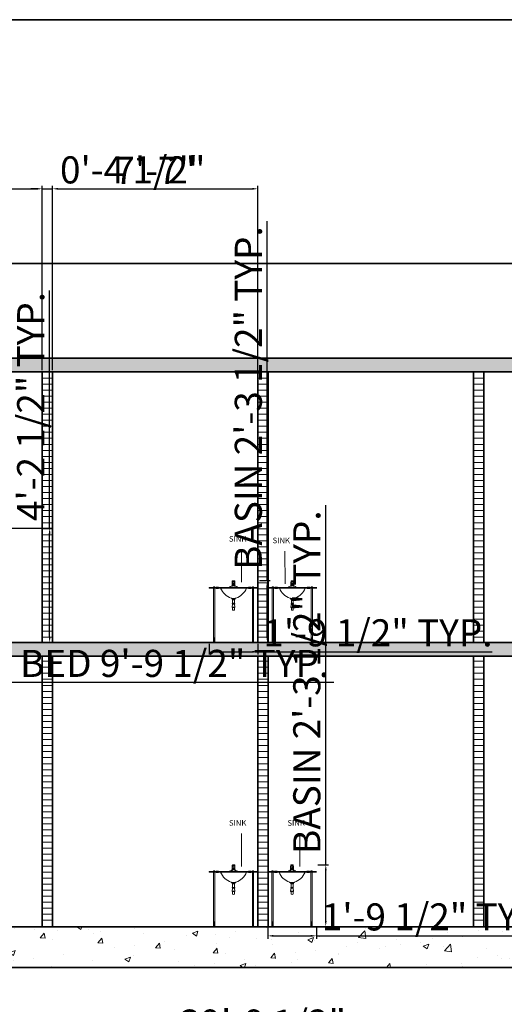
# Model space of a CAD drawing. Units: inches. Extents: x 2142 to 3604, y 1690 to 2981.
# Tile 8 of 9: x 3054 to 3269, y 2545 to 2981. Entities that reach past the tile are written whole.
import ezdxf

# ---------------------------------------------------------------- set-up
doc = ezdxf.new("R2010")
doc.units = ezdxf.units.IN
for name, color, linetype, lineweight in [('A-ANNO-DIMS', 2, 'Continuous', 18), ('A-ANNO-TEXT', 7, 'Continuous', 18), ('A-ANNO-TTLB', 7, 'Continuous', 35), ('A-FLOR-FIXT', 8, 'Continuous', 18), ('A-FLOR-PATT', 8, 'Continuous', 13), ('A-SECT', 7, 'Continuous', 35), ('A-WALL-PATT', 8, 'Continuous', 13)]:
    doc.layers.add(name, color=color, linetype=linetype, lineweight=lineweight)
doc.styles.get("Standard").update_dxf_attribs({"font": 'arial.ttf'})
doc.dimstyles.new('ISO-25', dxfattribs={"dimtxt": 12, "dimasz": 2.5, "dimexe": 1.25, "dimexo": 0.625, "dimtad": 1, "dimdec": 0, "dimlunit": 3, "dimtxsty": 'Standard', "dimcen": 2.5, "dimadec": 0, "dimazin": 0, "dimtfac": 1, "dimtdec": 0, "dimtmove": 0, "dimatfit": 3, "dimfxl": 1, "dimarcsym": 0})

# ---------------------------------------------------------------- blocks, each defined once
blk = doc.blocks.new('BASIN-STAND-UPPER')
for p, q in [((10.2, 27.18), (10.14, 26.52)), ((10.19, 26.42), (10.14, 26.34)), ((10.22, 25.79), (10.22, 26.23)), ((10.22, 26.23), (10.22, 25.79)), ((11.29, 26.23), (11.29, 25.79)), ((11.37, 26.52), (11.31, 27.18)), ((11.37, 26.34), (11.32, 26.42)), ((21.58, 24.41), (0, 24.41)), ((0, 24.41), (0, 24.07)), ((0, 24.07), (21.58, 24.07)), ((2.43, 24.7), (1.85, 24.7)), ((1.85, 24.7), (1.85, 24.41)), ((1.85, 0), (1.85, 24.07)), ((2.43, 24.41), (2.43, 24.7)), ((2.43, 0), (2.43, 24.07)), ((3, 24.41), (3, 24.56)), ((3, 24.56), (4.15, 24.56)), ((3, 23.93), (3, 24.07)), ((4.15, 23.93), (3, 23.93)), ((4.15, 24.56), (4.15, 24.41)), ((4.15, 24.07), (4.15, 23.93)), ((9.15, 24.64), (9.14, 24.41)), ((9.14, 24.41), (12.37, 24.41)), ((9.82, 24.89), (9.26, 24.77)), ((9.82, 24.89), (10.09, 24.92)), ((10.32, 25.11), (10.34, 25.4)), ((10.5, 25.55), (11.01, 25.55)), ((10.53, 25.36), (10.53, 25.22)), ((10.98, 25.22), (10.98, 25.36)), ((11.17, 25.4), (11.19, 25.11)), ((11.42, 24.92), (11.69, 24.89)), ((12.25, 24.77), (11.69, 24.89)), ((12.37, 24.41), (12.36, 24.64)), ((18.51, 24.56), (17.36, 24.56)), ((17.36, 24.56), (17.36, 24.41)), ((17.36, 24.07), (17.36, 23.93)), ((17.36, 23.93), (18.51, 23.93)), ((18.51, 24.41), (18.51, 24.56)), ((18.51, 23.93), (18.51, 24.07)), ((19.66, 24.7), (19.08, 24.7)), ((19.08, 24.7), (19.08, 24.41)), ((19.08, 0), (19.08, 24.07)), ((19.66, 24.41), (19.66, 24.7)), ((19.66, 0), (19.66, 24.07)), ((10, 19.49), (10.16, 19.49)), ((10.16, 19.49), (11.51, 19.49)), ((10.16, 19.33), (11.35, 19.33)), ((10.16, 19.33), (10.16, 19.1)), ((10.16, 19.1), (11.35, 19.1)), ((10.32, 18.93), (11.19, 18.93)), ((10.32, 18.93), (10.32, 17.35)), ((11.19, 17.35), (11.19, 18.93)), ((11.35, 19.1), (11.35, 19.33)), ((10.32, 16.95), (10.12, 15.64)), ((10.12, 15.64), (11.39, 15.64)), ((10.32, 17.35), (10.3, 17.35)), ((10.3, 17.18), (11.21, 17.18)), ((10.3, 17.18), (10.3, 17.12)), ((10.3, 17.12), (11.21, 17.12)), ((10.3, 16.95), (10.32, 16.95)), ((10.32, 17.35), (11.19, 17.35)), ((10.32, 16.95), (11.19, 16.95)), ((10.32, 15.52), (11.19, 15.52)), ((10.32, 15.52), (10.32, 14.33)), ((11.21, 17.35), (11.19, 17.35)), ((11.39, 15.64), (11.19, 16.95)), ((11.19, 16.95), (11.21, 16.95)), ((11.19, 14.33), (11.19, 15.52)), ((11.21, 17.12), (11.21, 17.18)), ((1.88, 1.8), (1.88, 0)), ((1.94, 1.87), (1.94, 0)), ((2.01, 1.96), (2.01, 0)), ((2.1, 2.05), (2.1, 0)), ((2.24, 2.16), (2.24, 0)), ((19.11, 1.8), (19.11, 0)), ((19.17, 1.87), (19.17, 0)), ((19.25, 1.96), (19.25, 0)), ((19.34, 2.05), (19.34, 0)), ((19.48, 2.16), (19.48, 0))]:
    blk.add_line(p, q)
for centre, radius, start, end in [((-23.87, 27.85), 34.05, 355.4804, 357.4686), ((10.59, 26.7), 0.482, 202.3486, 215.3932), ((10.75, 29.15), 2.87, 257.6538, 282.3462), ((10.75, 28.35), 2, 253.7222, 286.2778), ((10.34, 27.17), 0.144, 109.5533, 175.0912), ((12.7, 26.18), 2.5, 160.4627, 171.5377), ((10.22, 28.02), 0.772, 272.2221, 297.8083), ((10.75, 26), 1.38, 70.4555, 109.5445), ((10.71, 26.93), 0.376, 125.1003, 167.0073), ((10.66, 26.94), 0.265, 108.5012, 184.1781), ((10.75, 27.75), 0.908, 246.8267, 293.1733), ((10.55, 27.03), 0.222, 76.2618, 106.2494), ((10.75, 26.49), 0.861, 78.0249, 101.9751), ((10.77, 28.74), 1.56, 262.99, 275.8762), ((10.75, 28.01), 0.785, 258.9912, 281.0088), ((10.96, 27.03), 0.222, 73.7506, 103.7382), ((11.29, 28.02), 0.772, 242.1917, 267.7779), ((10.85, 26.94), 0.265, 355.8219, 71.4988), ((10.8, 26.93), 0.376, 12.9927, 54.8997), ((8.81, 26.18), 2.5, 8.4623, 19.5373), ((11.17, 27.17), 0.144, 4.9088, 70.4467), ((10.92, 26.7), 0.482, 324.6068, 337.6514), ((45.38, 27.85), 34.05, 182.5314, 184.5196), ((12.33, 27.15), 7.95, 202.8132, 250.4339), ((9.29, 24.63), 0.144, 101.5368, 177.9892), ((9.77, 25.18), 0.298, 279.2684, 356.7643), ((10.04, 25.2), 0.29, 279.6116, 341.5359), ((10.29, 25.78), 0.0636, 174.5586, 276.0081), ((10.27, 26.1), 0.375, 273.4496, 304.987), ((10.54, 25.35), 0.202, 102.2181, 166.3983), ((10.75, 24.82), 1.01, 74.5269, 105.4731), ((10.75, 25.06), 0.372, 52.7942, 127.2058), ((10.97, 25.35), 0.202, 13.6017, 77.7819), ((11.24, 26.1), 0.375, 235.013, 266.5504), ((11.47, 25.2), 0.29, 198.4641, 260.3884), ((11.22, 25.78), 0.0636, 263.9919, 5.4414), ((11.74, 25.18), 0.298, 183.2357, 260.7316), ((9.18, 27.15), 7.95, 289.5661, 337.1868), ((12.22, 24.63), 0.144, 2.0108, 78.4632), ((9.28, 18.51), 1.22, 53.5473, 71.0224), ((10.49, 19.82), 0.59, 213.8308, 236.15), ((10.6, 19.35), 0.507, 209.6921, 236.6714), ((10.75, 17.21), 0.574, 138.5904, 218.9808), ((10.91, 19.35), 0.507, 303.3286, 330.3079), ((10.75, 17.21), 0.574, 321.0192, 41.4096), ((11.02, 19.82), 0.59, 303.85, 326.1692), ((12.23, 18.51), 1.22, 108.9776, 126.4527), ((10.33, 15.78), 0.253, 212.9626, 267.5476), ((10.33, 17.26), 0.0933, 112.6199, 247.3801), ((10.33, 17.03), 0.0933, 112.6199, 247.3801), ((10.75, 15.92), 1.64, 254.8107, 285.1893), ((11.17, 15.78), 0.253, 272.4524, 327.0374), ((11.18, 17.26), 0.0933, 292.6199, 67.3801), ((11.18, 17.03), 0.0933, 292.6199, 67.3801), ((3.1, 0.95), 1.49, 117.0595, 147.278), ((20.34, 0.95), 1.49, 117.0595, 147.278)]:
    blk.add_arc(centre, radius, start, end)
blk.add_ellipse((10.75, 25.22), major_axis=(0.225, 0), ratio=0.294234)
blk = doc.blocks.new('BASIN-STAND-LOWER')
for p, q in [((10.2, 27.18), (10.14, 26.52)), ((10.19, 26.42), (10.14, 26.34)), ((10.22, 25.79), (10.22, 26.23)), ((10.22, 26.23), (10.22, 25.79)), ((11.29, 26.23), (11.29, 25.79)), ((11.37, 26.52), (11.31, 27.18)), ((11.37, 26.34), (11.32, 26.42)), ((21.58, 24.41), (0, 24.41)), ((0, 24.41), (0, 24.07)), ((0, 24.07), (21.58, 24.07)), ((2.43, 24.7), (1.85, 24.7)), ((1.85, 24.7), (1.85, 24.41)), ((1.85, 0), (1.85, 24.07)), ((2.43, 24.41), (2.43, 24.7)), ((2.43, 0), (2.43, 24.07)), ((3, 24.41), (3, 24.56)), ((3, 24.56), (4.15, 24.56)), ((3, 23.93), (3, 24.07)), ((4.15, 23.93), (3, 23.93)), ((4.15, 24.56), (4.15, 24.41)), ((4.15, 24.07), (4.15, 23.93)), ((9.15, 24.64), (9.14, 24.41)), ((9.14, 24.41), (12.37, 24.41)), ((9.82, 24.89), (9.26, 24.77)), ((9.82, 24.89), (10.09, 24.92)), ((10.32, 25.11), (10.34, 25.4)), ((10.5, 25.55), (11.01, 25.55)), ((10.53, 25.36), (10.53, 25.22)), ((10.98, 25.22), (10.98, 25.36)), ((11.17, 25.4), (11.19, 25.11)), ((11.42, 24.92), (11.69, 24.89)), ((12.25, 24.77), (11.69, 24.89)), ((12.37, 24.41), (12.36, 24.64)), ((18.51, 24.56), (17.36, 24.56)), ((17.36, 24.56), (17.36, 24.41)), ((17.36, 24.07), (17.36, 23.93)), ((17.36, 23.93), (18.51, 23.93)), ((18.51, 24.41), (18.51, 24.56)), ((18.51, 23.93), (18.51, 24.07)), ((19.66, 24.7), (19.08, 24.7)), ((19.08, 24.7), (19.08, 24.41)), ((19.08, 0), (19.08, 24.07)), ((19.66, 24.41), (19.66, 24.7)), ((19.66, 0), (19.66, 24.07)), ((10, 19.49), (10.16, 19.49)), ((10.16, 19.49), (11.51, 19.49)), ((10.16, 19.33), (11.35, 19.33)), ((10.16, 19.33), (10.16, 19.1)), ((10.16, 19.1), (11.35, 19.1)), ((10.32, 18.93), (11.19, 18.93)), ((10.32, 18.93), (10.32, 17.35)), ((11.19, 17.35), (11.19, 18.93)), ((11.35, 19.1), (11.35, 19.33)), ((10.32, 16.95), (10.12, 15.64)), ((10.12, 15.64), (11.39, 15.64)), ((10.32, 17.35), (10.3, 17.35)), ((10.3, 17.18), (11.21, 17.18)), ((10.3, 17.18), (10.3, 17.12)), ((10.3, 17.12), (11.21, 17.12)), ((10.3, 16.95), (10.32, 16.95)), ((10.32, 17.35), (11.19, 17.35)), ((10.32, 16.95), (11.19, 16.95)), ((10.32, 15.52), (11.19, 15.52)), ((10.32, 15.52), (10.32, 14.33)), ((11.21, 17.35), (11.19, 17.35)), ((11.39, 15.64), (11.19, 16.95)), ((11.19, 16.95), (11.21, 16.95)), ((11.19, 14.33), (11.19, 15.52)), ((11.21, 17.12), (11.21, 17.18)), ((2.24, 2.16), (2.24, 0)), ((19.48, 2.16), (19.48, 0))]:
    blk.add_line(p, q)
for centre, radius, start, end in [((-23.87, 27.85), 34.05, 355.4804, 357.4686), ((10.59, 26.7), 0.482, 202.3486, 215.3932), ((10.75, 29.15), 2.87, 257.6538, 282.3462), ((10.75, 28.35), 2, 253.7222, 286.2778), ((10.34, 27.17), 0.144, 109.5533, 175.0912), ((12.7, 26.18), 2.5, 160.4627, 171.5377), ((10.22, 28.02), 0.772, 272.2221, 297.8083), ((10.75, 26), 1.38, 70.4555, 109.5445), ((10.71, 26.93), 0.376, 125.1003, 167.0073), ((10.66, 26.94), 0.265, 108.5012, 184.1781), ((10.75, 27.75), 0.908, 246.8267, 293.1733), ((10.55, 27.03), 0.222, 76.2618, 106.2494), ((10.75, 26.49), 0.861, 78.0249, 101.9751), ((10.77, 28.74), 1.56, 262.99, 275.8762), ((10.75, 28.01), 0.785, 258.9912, 281.0088), ((10.96, 27.03), 0.222, 73.7506, 103.7382), ((11.29, 28.02), 0.772, 242.1917, 267.7779), ((10.85, 26.94), 0.265, 355.8219, 71.4988), ((10.8, 26.93), 0.376, 12.9927, 54.8997), ((8.81, 26.18), 2.5, 8.4623, 19.5373), ((11.17, 27.17), 0.144, 4.9088, 70.4467), ((10.92, 26.7), 0.482, 324.6068, 337.6514), ((45.38, 27.85), 34.05, 182.5314, 184.5196), ((12.33, 27.15), 7.95, 202.8132, 250.4339), ((9.29, 24.63), 0.144, 101.5368, 177.9892), ((9.77, 25.18), 0.298, 279.2684, 356.7643), ((10.04, 25.2), 0.29, 279.6116, 341.5359), ((10.29, 25.78), 0.0636, 174.5586, 276.0081), ((10.27, 26.1), 0.375, 273.4496, 304.987), ((10.54, 25.35), 0.202, 102.2181, 166.3983), ((10.75, 24.82), 1.01, 74.5269, 105.4731), ((10.75, 25.06), 0.372, 52.7942, 127.2058), ((10.97, 25.35), 0.202, 13.6017, 77.7819), ((11.24, 26.1), 0.375, 235.013, 266.5504), ((11.47, 25.2), 0.29, 198.4641, 260.3884), ((11.22, 25.78), 0.0636, 263.9919, 5.4414), ((11.74, 25.18), 0.298, 183.2357, 260.7316), ((9.18, 27.15), 7.95, 289.5661, 337.1868), ((12.22, 24.63), 0.144, 2.0108, 78.4632), ((9.28, 18.51), 1.22, 53.5473, 71.0224), ((10.49, 19.82), 0.59, 213.8308, 236.15), ((10.6, 19.35), 0.507, 209.6921, 236.6714), ((10.75, 17.2), 0.574, 138.5904, 218.9808), ((10.91, 19.35), 0.507, 303.3286, 330.3079), ((10.75, 17.2), 0.574, 321.0192, 41.4096), ((11.02, 19.82), 0.59, 303.85, 326.1692), ((12.23, 18.51), 1.22, 108.9776, 126.4527), ((10.33, 15.78), 0.253, 212.9626, 267.5476), ((10.33, 17.26), 0.0933, 112.6199, 247.3801), ((10.33, 17.03), 0.0933, 112.6199, 247.3801), ((10.75, 15.92), 1.64, 254.8107, 285.1893), ((11.17, 15.78), 0.253, 272.4524, 327.0374), ((11.18, 17.26), 0.0933, 292.6199, 67.3801), ((11.18, 17.03), 0.0933, 292.6199, 67.3801), ((3.1, 0.95), 1.49, 117.0595, 147.278), ((20.34, 0.95), 1.49, 117.0595, 147.278)]:
    blk.add_arc(centre, radius, start, end)
blk.add_ellipse((10.75, 25.22), major_axis=(0.225, 0), ratio=0.294234)
blk = doc.blocks.new('*D41')
at = {"layer": 'A-ANNO-DIMS', "color": 0, "lineweight": -2, "transparency": 16777216}
for p, q in [((2932.33, 2704.39), (2932.33, 2686.12)), ((3049.95, 2704.39), (3049.95, 2686.12)), ((2934.83, 2687.37), (3047.45, 2687.37)), ((3049.95, 2687.37), (3193.4, 2687.37))]:
    blk.add_line(p, q, dxfattribs=at)
at = {"layer": 'A-ANNO-DIMS', "color": 0, "transparency": 16777216}
for points in [[(2934.83, 2687.79), (2934.83, 2686.96), (2932.33, 2687.37)], [(3047.45, 2687.79), (3047.45, 2686.96), (3049.95, 2687.37)]]:
    blk.add_solid(points, dxfattribs=at)
at = {"layer": 'Defpoints', "color": 0, "transparency": 16777216}
for p in [(2932.33, 2705.02), (3049.95, 2705.02), (3049.95, 2687.37)]:
    blk.add_point(p, dxfattribs=at)
at = {"layer": 'A-ANNO-DIMS', "color": 0, "transparency": 16777216, "insert": (3122.93, 2694.2), "char_height": 12, "attachment_point": 5}
blk.add_mtext('BED 9\'-9 1/2" TYP.', dxfattribs=at)
blk = doc.blocks.new('*D42')
at = {"layer": 'A-ANNO-DIMS', "color": 0, "lineweight": -2, "transparency": 16777216}
for p, q in [((3067.59, 2755.67), (3067.59, 2861.01)), ((3050.58, 2755.67), (3068.84, 2755.67)), ((3067.59, 2707.52), (3067.59, 2753.17)), ((3050.58, 2705.02), (3068.84, 2705.02))]:
    blk.add_line(p, q, dxfattribs=at)
at = {"layer": 'A-ANNO-DIMS', "color": 0, "transparency": 16777216}
for points in [[(3067.18, 2753.17), (3068.01, 2753.17), (3067.59, 2755.67)], [(3067.18, 2707.52), (3068.01, 2707.52), (3067.59, 2705.02)]]:
    blk.add_solid(points, dxfattribs=at)
at = {"layer": 'Defpoints', "color": 0, "transparency": 16777216}
for p in [(3049.95, 2755.67), (3067.59, 2755.67), (3049.95, 2705.02)]:
    blk.add_point(p, dxfattribs=at)
at = {"layer": 'A-ANNO-DIMS', "color": 0, "transparency": 16777216, "insert": (3060.76, 2809.59), "char_height": 12, "attachment_point": 5, "rotation": 90}
blk.add_mtext('4\'-2 1/2" TYP.', dxfattribs=at)
blk = doc.blocks.new('*D73')
at = {"layer": 'A-ANNO-DIMS', "color": 0, "lineweight": -2, "transparency": 16777216}
for p, q in [((3163.94, 2732.43), (3163.94, 2891.72)), ((3160.46, 2732.43), (3165.19, 2732.43)), ((3163.94, 2707.52), (3163.94, 2729.93)), ((3160.46, 2705.02), (3165.19, 2705.02))]:
    blk.add_line(p, q, dxfattribs=at)
at = {"layer": 'A-ANNO-DIMS', "color": 0, "transparency": 16777216}
for points in [[(3163.53, 2729.93), (3164.36, 2729.93), (3163.94, 2732.43)], [(3163.53, 2707.52), (3164.36, 2707.52), (3163.94, 2705.02)]]:
    blk.add_solid(points, dxfattribs=at)
at = {"layer": 'Defpoints', "color": 0, "transparency": 16777216}
for p in [(3159.83, 2732.43), (3163.94, 2732.43), (3159.83, 2705.02)]:
    blk.add_point(p, dxfattribs=at)
at = {"layer": 'A-ANNO-DIMS', "color": 0, "transparency": 16777216, "insert": (3157.11, 2813.32), "char_height": 12, "attachment_point": 5, "rotation": 90}
blk.add_mtext('BASIN 2\'-3 1/2" TYP.', dxfattribs=at)
blk = doc.blocks.new('*D74')
at = {"layer": 'A-ANNO-DIMS', "color": 0, "lineweight": -2, "transparency": 16777216}
for p, q in [((3138.26, 2704.39), (3138.26, 2699.66)), ((3159.83, 2704.39), (3159.83, 2699.66)), ((3140.76, 2700.91), (3157.33, 2700.91)), ((3159.83, 2700.91), (3263.56, 2700.91))]:
    blk.add_line(p, q, dxfattribs=at)
at = {"layer": 'A-ANNO-DIMS', "color": 0, "transparency": 16777216}
for points in [[(3140.76, 2701.32), (3140.76, 2700.49), (3138.26, 2700.91)], [(3157.33, 2701.32), (3157.33, 2700.49), (3159.83, 2700.91)]]:
    blk.add_solid(points, dxfattribs=at)
at = {"layer": 'Defpoints', "color": 0, "transparency": 16777216}
for p in [(3138.26, 2705.02), (3159.83, 2705.02), (3159.83, 2700.91)]:
    blk.add_point(p, dxfattribs=at)
at = {"layer": 'A-ANNO-DIMS', "color": 0, "transparency": 16777216, "insert": (3212.95, 2707.74), "char_height": 12, "attachment_point": 5}
blk.add_mtext('1\'-9 1/2" TYP.', dxfattribs=at)
blk = doc.blocks.new('*D75')
at = {"layer": 'A-ANNO-DIMS', "color": 0, "lineweight": -2, "transparency": 16777216}
for p, q in [((3189.85, 2606.53), (3189.85, 2765.82)), ((3186.36, 2606.53), (3191.1, 2606.53)), ((3189.85, 2581.62), (3189.85, 2604.03)), ((3186.36, 2579.12), (3191.1, 2579.12))]:
    blk.add_line(p, q, dxfattribs=at)
at = {"layer": 'A-ANNO-DIMS', "color": 0, "transparency": 16777216}
for points in [[(3189.43, 2604.03), (3190.26, 2604.03), (3189.85, 2606.53)], [(3189.43, 2581.62), (3190.26, 2581.62), (3189.85, 2579.12)]]:
    blk.add_solid(points, dxfattribs=at)
at = {"layer": 'Defpoints', "color": 0, "transparency": 16777216}
for p in [(3185.73, 2606.53), (3189.85, 2606.53), (3185.73, 2579.12)]:
    blk.add_point(p, dxfattribs=at)
at = {"layer": 'A-ANNO-DIMS', "color": 0, "transparency": 16777216, "insert": (3183.01, 2687.43), "char_height": 12, "attachment_point": 5, "rotation": 90}
blk.add_mtext('BASIN 2\'-3 1/2" TYP.', dxfattribs=at)
blk = doc.blocks.new('*D76')
at = {"layer": 'A-ANNO-DIMS', "color": 0, "lineweight": -2, "transparency": 16777216}
for p, q in [((3164.16, 2578.5), (3164.16, 2573.76)), ((3166.66, 2575.01), (3183.23, 2575.01)), ((3185.73, 2578.5), (3185.73, 2573.76)), ((3185.73, 2575.01), (3289.46, 2575.01))]:
    blk.add_line(p, q, dxfattribs=at)
at = {"layer": 'A-ANNO-DIMS', "color": 0, "transparency": 16777216}
for points in [[(3166.66, 2575.43), (3166.66, 2574.59), (3164.16, 2575.01)], [(3183.23, 2575.43), (3183.23, 2574.59), (3185.73, 2575.01)]]:
    blk.add_solid(points, dxfattribs=at)
at = {"layer": 'Defpoints', "color": 0, "transparency": 16777216}
for p in [(3164.16, 2579.12), (3185.73, 2579.12), (3185.73, 2575.01)]:
    blk.add_point(p, dxfattribs=at)
at = {"layer": 'A-ANNO-DIMS', "color": 0, "transparency": 16777216, "insert": (3238.85, 2581.84), "char_height": 12, "attachment_point": 5}
blk.add_mtext('1\'-9 1/2" TYP.', dxfattribs=at)
blk = doc.blocks.new('*D93')
at = {"layer": 'A-ANNO-DIMS', "color": 0, "lineweight": -2, "transparency": 16777216}
for p, q in [((2923.33, 2560.39), (2923.33, 2526.72)), ((3400.83, 2560.39), (3400.83, 2526.72)), ((2925.83, 2527.97), (3398.33, 2527.97))]:
    blk.add_line(p, q, dxfattribs=at)
at = {"layer": 'A-ANNO-DIMS', "color": 0, "transparency": 16777216}
for points in [[(2925.83, 2528.38), (2925.83, 2527.55), (2923.33, 2527.97)], [(3398.33, 2528.38), (3398.33, 2527.55), (3400.83, 2527.97)]]:
    blk.add_solid(points, dxfattribs=at)
at = {"layer": 'Defpoints', "color": 0, "transparency": 16777216}
for p in [(2923.33, 2561.02), (3400.83, 2561.02), (3400.83, 2527.97)]:
    blk.add_point(p, dxfattribs=at)
at = {"layer": 'A-ANNO-DIMS', "color": 0, "transparency": 16777216, "insert": (3162.08, 2534.8), "char_height": 12, "attachment_point": 5}
blk.add_mtext('39\'-9 1/2"', dxfattribs=at)
blk = doc.blocks.new('*D95')
at = {"layer": 'A-ANNO-DIMS', "color": 0, "lineweight": -2, "transparency": 16777216}
for p, q in [((2932.33, 2825.64), (2932.33, 2907.32)), ((2934.83, 2906.07), (3061.83, 2906.07)), ((3064.33, 2825.64), (3064.33, 2907.32))]:
    blk.add_line(p, q, dxfattribs=at)
at = {"layer": 'A-ANNO-DIMS', "color": 0, "transparency": 16777216}
for points in [[(2934.83, 2906.48), (2934.83, 2905.65), (2932.33, 2906.07)], [(3061.83, 2906.48), (3061.83, 2905.65), (3064.33, 2906.07)]]:
    blk.add_solid(points, dxfattribs=at)
at = {"layer": 'Defpoints', "color": 0, "transparency": 16777216}
for p in [(3064.33, 2906.07), (2932.33, 2825.02), (3064.33, 2825.02)]:
    blk.add_point(p, dxfattribs=at)
at = {"layer": 'A-ANNO-DIMS', "color": 0, "transparency": 16777216, "insert": (2998.33, 2912.82), "char_height": 12, "attachment_point": 5}
blk.add_mtext('11\'-0"', dxfattribs=at)
blk = doc.blocks.new('*D96')
at = {"layer": 'A-ANNO-DIMS', "color": 0, "lineweight": -2, "transparency": 16777216}
for p, q in [((3068.83, 2825.64), (3068.83, 2907.32)), ((3071.33, 2906.07), (3157.33, 2906.07)), ((3159.83, 2825.64), (3159.83, 2907.32))]:
    blk.add_line(p, q, dxfattribs=at)
at = {"layer": 'A-ANNO-DIMS', "color": 0, "transparency": 16777216}
for points in [[(3071.33, 2906.48), (3071.33, 2905.65), (3068.83, 2906.07)], [(3157.33, 2906.48), (3157.33, 2905.65), (3159.83, 2906.07)]]:
    blk.add_solid(points, dxfattribs=at)
at = {"layer": 'Defpoints', "color": 0, "transparency": 16777216}
for p in [(3159.83, 2906.07), (3068.83, 2825.02), (3159.83, 2825.02)]:
    blk.add_point(p, dxfattribs=at)
at = {"layer": 'A-ANNO-DIMS', "color": 0, "transparency": 16777216, "insert": (3114.33, 2912.69), "char_height": 12, "attachment_point": 5}
blk.add_mtext('7\'-7"', dxfattribs=at)
blk = doc.blocks.new('*D97')
at = {"layer": 'A-ANNO-DIMS', "color": 0, "lineweight": -2, "transparency": 16777216}
for p, q in [((3061.83, 2906.07), (3059.33, 2906.07)), ((3064.33, 2825.64), (3064.33, 2907.32)), ((3064.33, 2906.07), (3068.83, 2906.07)), ((3068.83, 2825.64), (3068.83, 2907.32)), ((3071.33, 2906.07), (3134.94, 2906.07))]:
    blk.add_line(p, q, dxfattribs=at)
at = {"layer": 'A-ANNO-DIMS', "color": 0, "transparency": 16777216}
for points in [[(3061.83, 2906.48), (3061.83, 2905.65), (3064.33, 2906.07)], [(3071.33, 2906.48), (3071.33, 2905.65), (3068.83, 2906.07)]]:
    blk.add_solid(points, dxfattribs=at)
at = {"layer": 'Defpoints', "color": 0, "transparency": 16777216}
for p in [(3068.83, 2906.07), (3064.33, 2825.02), (3068.83, 2825.02)]:
    blk.add_point(p, dxfattribs=at)
at = {"layer": 'A-ANNO-DIMS', "color": 0, "transparency": 16777216, "insert": (3104.39, 2912.9), "char_height": 12, "attachment_point": 5}
blk.add_mtext('0\'-4 1/2"', dxfattribs=at)

msp = doc.modelspace()

# ---------------------------------------------------------------- hatches: boundary and pattern name
at = {"layer": 'A-FLOR-PATT'}
h = msp.add_hatch(dxfattribs=at)
h.set_pattern_fill('AR-CONC', color=256, scale=0.065, style=0)
h.paths.add_polyline_path([(2923.33, 2825.02), (3400.83, 2825.02), (3400.83, 2831.02), (2923.33, 2831.02)])
h = msp.add_hatch(dxfattribs=at)
h.set_pattern_fill('AR-CONC', color=256, scale=0.065, style=0)
h.paths.add_polyline_path([(2923.33, 2699.02), (3400.83, 2699.02), (3400.83, 2705.02), (2923.33, 2705.02)])
h = msp.add_hatch(dxfattribs=at)
h.set_pattern_fill('AR-CONC', color=256, scale=0.14, style=0)
h.paths.add_polyline_path([(2923.33, 2561.02), (3400.83, 2561.02), (3400.83, 2579.02), (2923.33, 2579.02)])
at = {"layer": 'A-WALL-PATT'}
h = msp.add_hatch(dxfattribs=at)
h.set_pattern_fill('ANSI31', color=256, scale=0.840945, angle=-45, style=0)
h.paths.add_polyline_path([(3064.33, 2705.02), (3068.83, 2705.02), (3068.83, 2825.02), (3064.33, 2825.02)])
h = msp.add_hatch(dxfattribs=at)
h.set_pattern_fill('ANSI31', color=256, scale=0.840945, angle=-45, style=0)
h.paths.add_polyline_path([(3159.83, 2705.02), (3164.33, 2705.02), (3164.33, 2825.02), (3159.83, 2825.02)])
h = msp.add_hatch(dxfattribs=at)
h.set_pattern_fill('ANSI31', color=256, scale=0.840945, angle=-45, style=0)
h.paths.add_polyline_path([(3255.33, 2705.02), (3259.83, 2705.02), (3259.83, 2825.02), (3255.33, 2825.02)])
h = msp.add_hatch(dxfattribs=at)
h.set_pattern_fill('ANSI31', color=256, scale=0.840945, angle=-45, style=0)
h.paths.add_polyline_path([(3064.33, 2579.02), (3068.83, 2579.02), (3068.83, 2699.02), (3064.33, 2699.02)])
h = msp.add_hatch(dxfattribs=at)
h.set_pattern_fill('ANSI31', color=256, scale=0.840945, angle=-45, style=0)
h.paths.add_polyline_path([(3159.83, 2579.02), (3164.33, 2579.02), (3164.33, 2699.02), (3159.83, 2699.02)])
h = msp.add_hatch(dxfattribs=at)
h.set_pattern_fill('ANSI31', color=256, scale=0.840945, angle=-45, style=0)
h.paths.add_polyline_path([(3255.33, 2579.02), (3259.83, 2579.02), (3259.83, 2699.02), (3255.33, 2699.02)])

# ---------------------------------------------------------------- linework, layer by layer
at = {"layer": 'A-ANNO-TEXT'}
for p, q in [((3152.54, 2731.68), (3152.47, 2746.27)), ((3171.85, 2730.96), (3171.78, 2745.55)), ((3152.54, 2605.79), (3152.47, 2620.38)), ((3178.44, 2605.79), (3178.37, 2620.38))]:
    msp.add_line(p, q, dxfattribs=at)
at = {"layer": 'A-ANNO-TTLB'}
msp.add_lwpolyline([(2142.1, 2981.01), (3604.42, 2981.01), (3604.42, 1690.13), (2142.1, 1690.13)], close=True, dxfattribs=at)
at = {"layer": 'A-FLOR-FIXT'}
msp.add_line((3137.52, 2705.02), (3160.5, 2705.02), dxfattribs=at)
at = {"layer": 'A-SECT'}
for p, q in [((2923.33, 2873.02), (3400.83, 2873.02)), ((2923.33, 2831.02), (3400.83, 2831.02)), ((2923.33, 2825.02), (3400.83, 2825.02)), ((3064.33, 2825.02), (3064.33, 2705.02)), ((3068.83, 2825.02), (3068.83, 2705.02)), ((3159.83, 2825.02), (3159.83, 2705.02)), ((3164.29, 2825.02), (3164.29, 2705.02)), ((3255.33, 2825.02), (3255.33, 2705.02)), ((3259.83, 2825.02), (3259.83, 2705.02)), ((2923.33, 2705.02), (3400.83, 2705.02)), ((2923.33, 2699.02), (3400.83, 2699.02)), ((3064.33, 2699.02), (3064.33, 2579.02)), ((3068.83, 2699.02), (3068.83, 2579.02)), ((3159.83, 2699.02), (3159.83, 2579.02)), ((3164.29, 2699.02), (3164.29, 2579.02)), ((3255.33, 2699.02), (3255.33, 2579.02)), ((3259.83, 2699.02), (3259.83, 2579.02)), ((2923.33, 2579.02), (3400.83, 2579.02)), ((2923.33, 2561.02), (3400.83, 2561.02))]:
    msp.add_line(p, q, dxfattribs=at)

# ---------------------------------------------------------------- block references
at = {"layer": 'A-FLOR-FIXT'}
for name, p in [('BASIN-STAND-UPPER', (3138.26, 2705.02)), ('BASIN-STAND-UPPER', (3164.29, 2705.02)), ('BASIN-STAND-LOWER', (3138.26, 2579.12)), ('BASIN-STAND-LOWER', (3164.16, 2579.12))]:
    msp.add_blockref(name, p, dxfattribs=at)

# ---------------------------------------------------------------- texts
at = {"layer": 'A-ANNO-TEXT', "char_height": 2.5, "attachment_point": 1}
for insert in [(3146.99, 2752.2), (3166.3, 2751.48), (3146.99, 2626.3), (3172.89, 2626.3)]:
    msp.add_mtext_dynamic_manual_height_columns('SINK', width=49.4586, gutter_width=12.5, heights=[0], dxfattribs=dict(at, insert=insert))

# ---------------------------------------------------------------- dimensions: what is measured, and where the dimension line sits
at = {"layer": 'A-ANNO-DIMS'}
for base, p1, p2, picture, middle in [((3068.83, 2906.07), (3064.33, 2825.02), (3068.83, 2825.02), '*D97', (3104.39, 2912.9)), ((3064.33, 2906.07), (2932.33, 2825.02), (3064.33, 2825.02), '*D95', (2998.33, 2912.82)), ((3159.83, 2906.07), (3068.83, 2825.02), (3159.83, 2825.02), '*D96', (3114.33, 2912.69)), ((3400.83, 2527.97), (2923.33, 2561.02), (3400.83, 2561.02), '*D93', (3162.08, 2534.8))]:
    dim = msp.add_linear_dim(base=base, p1=p1, p2=p2, dimstyle='ISO-25', override={"dimdec": 1, "dimlfac": 1, "dimrnd": 0, "dimzin": 1, "dimdsep": 46, "dimlunit": 4, "dimfrac": 2}, dxfattribs=at)
    dim.commit()
    dim.dimension.update_dxf_attribs({"geometry": picture, "text_midpoint": middle})
for base, p1, p2, text, picture, middle in [((3163.94, 2732.43), (3159.83, 2705.02), (3159.83, 2732.43), 'BASIN <> TYP.', '*D73', (3157.11, 2813.32)), ((3067.5938, 2755.67), (3049.9511, 2705.0172), (3049.9511, 2755.67), '<> TYP.', '*D42', (3060.7641, 2809.5903)), ((3189.85, 2606.53), (3185.73, 2579.12), (3185.73, 2606.53), 'BASIN <> TYP.', '*D75', (3183.01, 2687.43))]:
    dim = msp.add_linear_dim(base=base, p1=p1, p2=p2, angle=90, text=text, dimstyle='ISO-25', override={"dimdec": 1, "dimlfac": 1, "dimrnd": 0, "dimzin": 1, "dimdsep": 46, "dimlunit": 4, "dimfrac": 2}, dxfattribs=at)
    dim.commit()
    dim.dimension.update_dxf_attribs({"geometry": picture, "text_midpoint": middle})
for base, p1, p2, text, picture, middle in [((3049.95, 2687.37), (2932.33, 2705.02), (3049.95, 2705.02), 'BED <> TYP.', '*D41', (3122.93, 2694.2)), ((3159.83, 2700.91), (3138.26, 2705.02), (3159.83, 2705.02), '<> TYP.', '*D74', (3212.95, 2707.74)), ((3185.73, 2575.01), (3164.16, 2579.12), (3185.73, 2579.12), '<> TYP.', '*D76', (3238.85, 2581.84))]:
    dim = msp.add_linear_dim(base=base, p1=p1, p2=p2, text=text, dimstyle='ISO-25', override={"dimdec": 1, "dimlfac": 1, "dimrnd": 0, "dimzin": 1, "dimdsep": 46, "dimlunit": 4, "dimfrac": 2}, dxfattribs=at)
    dim.commit()
    dim.dimension.update_dxf_attribs({"geometry": picture, "text_midpoint": middle})

doc.saveas('drawing.dxf')
